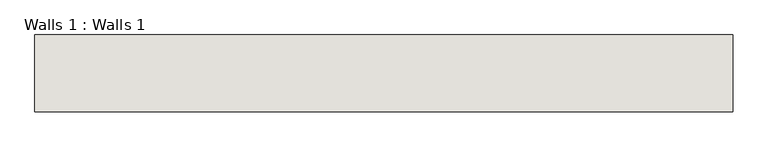
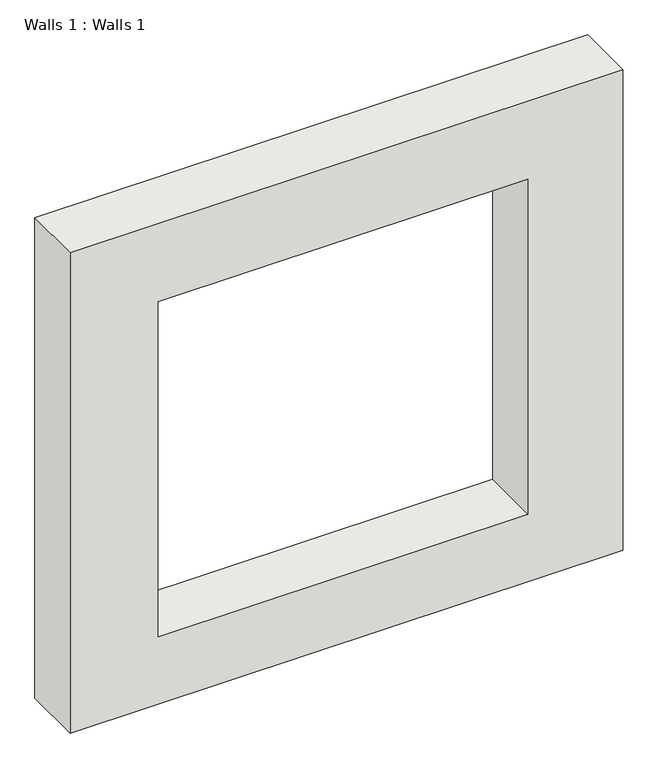
"""IFC4 building model written with IfcOpenShell, lengths in millimetres: wall geometry, Walls 1 : Walls 1."""

from ifc_helpers import new_model, si_unit, frame, origin, place, context, project, spatial, polyline, outline, extrude, source, transform, mapped, element, save


def walls_1_walls_1_b1444295(model_context):
    return source(origin(), model_context, "Body", "SweptSolid", [
        extrude(outline(polyline([(6981.9789316, -6069.6817469), (6981.9789316, -8558.8817469), (4695.9789316, -8558.8817469), (4695.9789316, -6069.6817469), (6981.9789316, -6069.6817469)]), holes=[polyline([(6610.4681256, -6498.1357575), (5016.6181256, -6498.1357575), (5016.6181256, -8161.8357575), (6610.4681256, -8161.8357575), (6610.4681256, -6498.1357575)])]), frame((0.0, 1408.0209854, 0.0), z_axis=(0.0, 1.0, 0.0), x_axis=(0.0, 0.0, 1.0)), (0.0, 0.0, 1.0), 274.2274628),
    ])


if __name__ == "__main__":
    model = new_model("IFC4")
    model_context = context("Model", 3, world=origin())
    ifc_project = project(units=[si_unit("LENGTHUNIT", "METRE", prefix="MILLI")], contexts=[model_context])
    site = spatial("IfcSite", under=ifc_project)
    building = spatial("IfcBuilding", under=site)
    placement = place(None, origin())
    walls_1_walls_1_shape = walls_1_walls_1_b1444295(model_context)
    element("IfcWall", 1, ObjectType="Walls 1 : Walls 1", at=placement, inside=building, context=model_context, shape_type="MappedRepresentation", body=[
        mapped(walls_1_walls_1_shape, transform((0.0, 0.0, 0.0), x_axis=(1.0, 0.0, 0.0), y_axis=(0.0, 1.0, 0.0), z_axis=(0.0, 0.0, 1.0))),
    ])
    save(model, "model.ifc")

# Revit data of these elements
# Element 1 (IfcWall, "Walls 1 : Walls 1")
#   Materials on its faces: "Default Wall"
# Materials
#   "Default Wall": colour RGB 128 128 128, transparency 0
